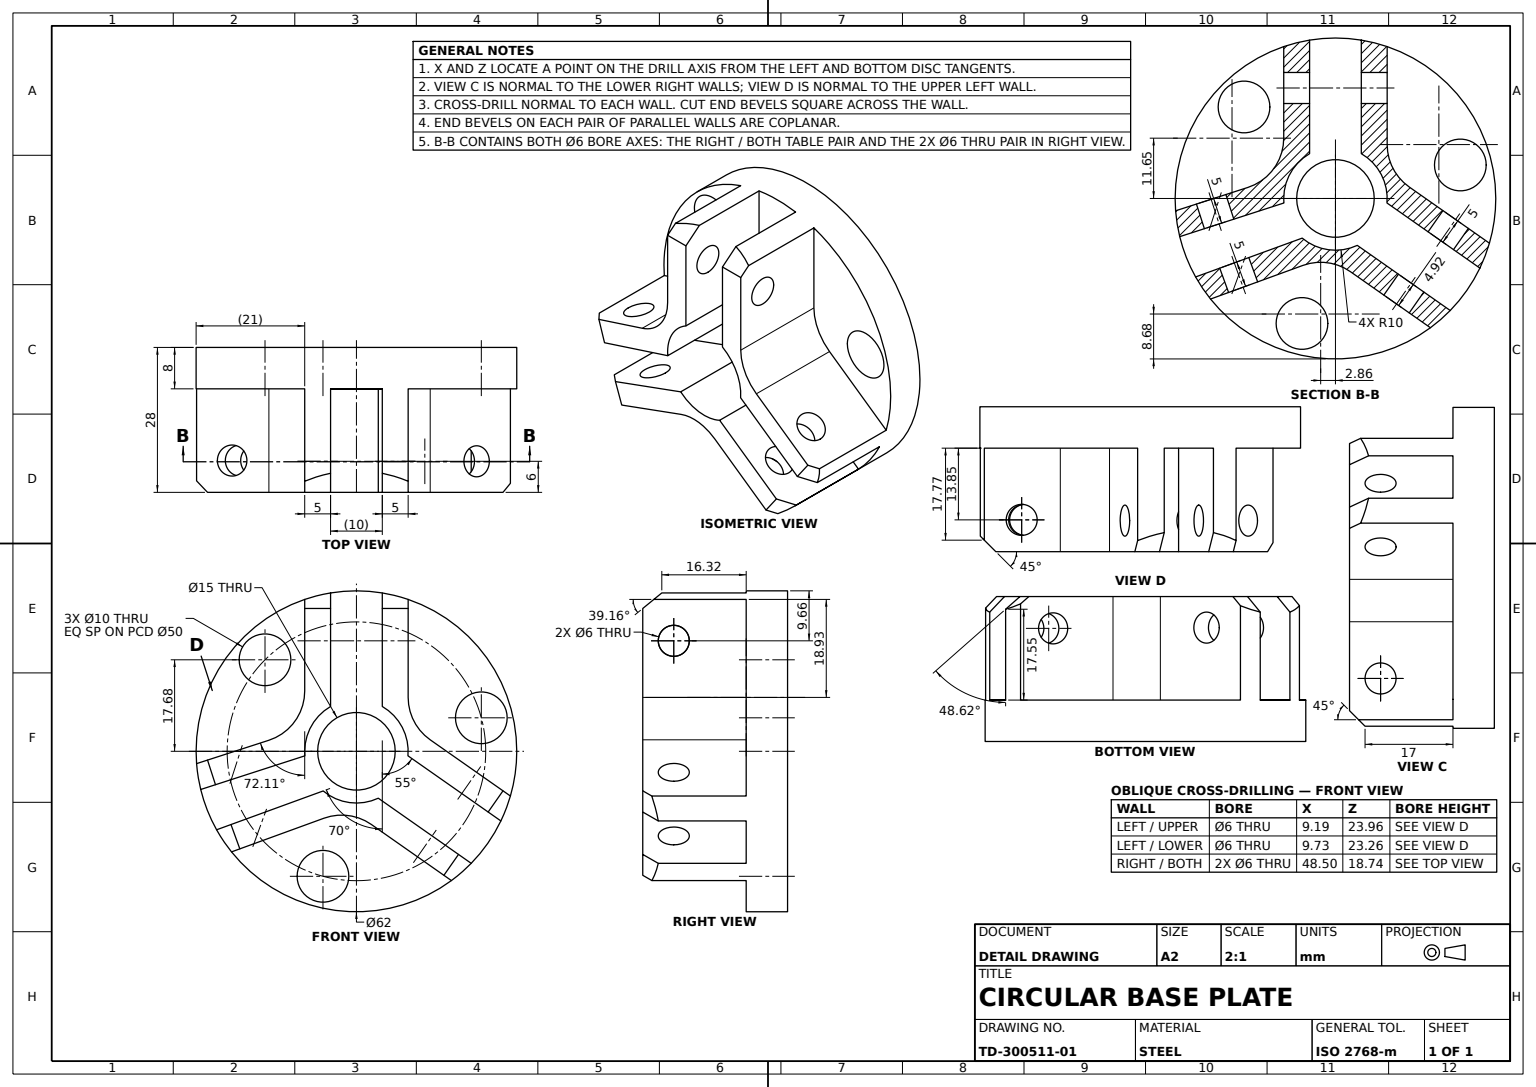
from build123d import *

# Parameters (mm, degrees)
BASE_DISC_SKETCH_R     = 31
BASE_DISC_62_DEPTH     = 8
SQUARE_CUT_SKETCH_R    = 5
SQUARE_CUT_10X10_DEPTH = 8
JAWS_DEPTH             = 20
JAW_NOTCH_1_DEPTH      = 10
JAW_NOTCH_2_DEPTH      = 10
JAW_NOTCH_3_DEPTH      = 10
JAW_NOTCH_4_DEPTH      = 10
JAW_NOTCH_5_DEPTH      = 10
JAW_NOTCH_6_DEPTH      = 10
JAW_HOLE_1_SKETCH_R    = 3
JAW_HOLE_1_6_DEPTH     = 10
JAW_HOLE_2_SKETCH_R    = 3
JAW_HOLE_2_6_DEPTH     = 10
JAW_HOLE_3_SKETCH_R    = 3
JAW_HOLE_3_6_DEPTH     = 10
JAW_START              = -10
JAW_HOLE_4_SKETCH_R    = 3
JAW_HOLE_4_6_DEPTH     = 10
JAW_HOLE_5_SKETCH_R    = 3
JAW_HOLE_5_6_DEPTH     = 10
JAW_HOLE_6_SKETCH_R    = 3
JAW_HOLE_6_6_DEPTH     = 10
HOLE_15_SKETCH_R       = 7.5
HOLE_15_DEPTH          = 10


with BuildPart() as part:
    # Base Disc Sketch → Base Disc Ø62 (new body)
    with BuildSketch(Plane.XY):
        Circle(BASE_DISC_SKETCH_R)
    extrude(amount=BASE_DISC_62_DEPTH)

    # Square Cut Sketch → Square Cut 10x10 (cut)
    with BuildSketch(Plane.XY.offset(8)):
        with Locations((-17.67766953, 17.67766953)):
            Circle(SQUARE_CUT_SKETCH_R)
        with Locations((24.148145657, 6.470476128)):
            Circle(SQUARE_CUT_SKETCH_R)
        with Locations((-6.470476128, -24.148145657)):
            Circle(SQUARE_CUT_SKETCH_R)
    extrude(amount=-SQUARE_CUT_10X10_DEPTH, mode=Mode.SUBTRACT)

    # Jaws Sketch → Jaws (add)
    with BuildSketch(Plane.XY.offset(8)):
        with BuildLine():
            Line((-30.109514993, -7.376795165), (-9.961946981, -0.871557427))
            ThreePointArc((-9.961946981, -0.871557427), (-9.990482216, 0.436193874), (-9.84807753, 1.736481777))
            ThreePointArc((-9.84807753, 1.736481777), (-8.191520443, 5.735764364), (-5, 8.660254038))
            Line((-5, 8.660254038), (-5, 10))
            Line((-5, 10), (-5, 30.594117082))
            ThreePointArc((-5, 30.594117082), (-7.526051267, 30.072554802), (-10, 29.342801502))
            Line((-10, 29.342801502), (-10, 11.649864154))
            ThreePointArc((-10, 11.649864154), (-11.915260032, 5.764545161), (-16.927395931, 2.133609416))
            Line((-16.927395931, 2.133609416), (-30.908458268, -2.38058973))
            ThreePointArc((-30.908458268, -2.38058973), (-30.611089207, -4.895019672), (-30.109514993, -7.376795165))
        make_face()
        with BuildLine():
            ThreePointArc((4.226182617, -9.06307787), (-1.305261922, -9.914448614), (-6.427876097, -7.660444431))
            Line((-6.427876097, -7.660444431), (-7.686825491, -8.118664537))
            Line((-7.686825491, -8.118664537), (-27.038965344, -15.162267413))
            ThreePointArc((-27.038965344, -15.162267413), (-25.684896703, -17.357594343), (-24.153012612, -19.432755383))
            Line((-24.153012612, -19.432755383), (-6.276119738, -12.926098496))
            ThreePointArc((-6.276119738, -12.926098496), (-1.550656383, -12.40857609), (2.879846058, -14.131504261))
            Line((2.879846058, -14.131504261), (18.365137045, -24.974421741))
            ThreePointArc((18.365137045, -24.974421741), (20.347505117, -23.387582934), (22.193351369, -21.64382487))
            Line((22.193351369, -21.64382487), (5.323638261, -9.831524585))
            Line((5.323638261, -9.831524585), (4.226182617, -9.06307787))
        make_face()
        with BuildLine():
            ThreePointArc((10, 29.342801502), (7.526051267, 30.072554802), (5, 30.594117082))
            Line((5, 30.594117082), (5, 10))
            Line((5, 10), (5, 8.660254038))
            ThreePointArc((5, 8.660254038), (8.870108332, 4.617486132), (9.961946981, -0.871557427))
            Line((9.961946981, -0.871557427), (11.059402625, -1.640004142))
            Line((11.059402625, -1.640004142), (27.929115732, -13.452304428))
            ThreePointArc((27.929115732, -13.452304428), (28.950760409, -11.083928535), (29.771980199, -8.638819075))
            Line((29.771980199, -8.638819075), (14.264235636, 2.219820568))
            ThreePointArc((14.264235636, 2.219820568), (11.129891668, 5.793854879), (10, 10.411341011))
            Line((10, 10.411341011), (10, 29.342801502))
        make_face()
    extrude(amount=JAWS_DEPTH)

    # Jaw Notch 1 Sketch → Jaw Notch 1 (cut)
    with BuildSketch(Plane.ZY.offset(-5)):
        Polygon((28, 30.594117082), (28, 27.594117082), (24.316442961, 30.594117082), align=None)
    extrude(amount=-JAW_NOTCH_1_DEPTH, mode=Mode.SUBTRACT)

    # Jaw Notch 2 Sketch → Jaw Notch 2 (cut)
    with BuildSketch(Plane(origin=(-5, 0, 0), x_dir=(0, 0, -1), z_dir=(1, 0, 0))):
        Polygon((-28, 30.594117082), (-24.316442961, 30.594117082), (-28, 27.594117082), align=None)
    extrude(amount=-JAW_NOTCH_2_DEPTH, mode=Mode.SUBTRACT)

    # Jaw Notch 3 Sketch → Jaw Notch 3 (cut)
    with BuildSketch(Plane(origin=(2.867882182, 4.095760221, 0), x_dir=(0.8191520442889944, -0.5735764363510426, 0), z_dir=(-0.5735764363510426, -0.8191520442889944, 0))):
        Polygon((30.594117082, 28), (30.594117082, 25), (27.594117082, 28), align=None)
    extrude(amount=-JAW_NOTCH_3_DEPTH, mode=Mode.SUBTRACT)

    # Jaw Notch 4 Sketch → Jaw Notch 4 (cut)
    with BuildSketch(Plane(origin=(-2.867882182, -4.095760221, 0), x_dir=(0.8191520442889944, -0.5735764363510426, 0), z_dir=(0.5735764363510426, 0.8191520442889944, 0))):
        Polygon((27.594117082, -28), (30.594117082, -28), (30.594117082, -25), align=None)
    extrude(amount=-JAW_NOTCH_4_DEPTH, mode=Mode.SUBTRACT)

    # Jaw Notch 5 Sketch → Jaw Notch 5 (cut)
    with BuildSketch(Plane(origin=(-0.685656401, 2.123567121, 0), x_dir=(0.9516254737982698, 0.3072604068509618, 0), z_dir=(0.3072604068509618, -0.9516254737982698, 0))):
        Polygon((-30.919578554, 28), (-27.919578554, 28), (-30.919578554, 25), align=None)
    extrude(amount=-JAW_NOTCH_5_DEPTH, mode=Mode.SUBTRACT)

    # Jaw Notch 6 Sketch → Jaw Notch 6 (cut)
    with BuildSketch(Plane(origin=(1.710100717, -4.698463104, 0), x_dir=(0.9396926207859072, 0.34202014332567215, 0), z_dir=(-0.3420201433256721, 0.9396926207859071, 0))):
        Polygon((-27.635003822, -28), (-30.594117082, -25.550278158), (-30.594117082, -28), align=None)
    extrude(amount=-JAW_NOTCH_6_DEPTH, mode=Mode.SUBTRACT)

    # Jaw Hole 1 Sketch → Jaw Hole 1 Ø6 (cut)
    with BuildSketch(Plane(origin=(-0.685656401, 2.123567121, 0), x_dir=(0.9516254737982698, 0.3072604068509618, 0), z_dir=(0.3072604068509618, -0.9516254737982698, 0))):
        with Locations((-22.919578554, 21.853934113)):
            Circle(JAW_HOLE_1_SKETCH_R)
    extrude(amount=-JAW_HOLE_1_6_DEPTH, mode=Mode.SUBTRACT)

    # Jaw Hole 2 Sketch → Jaw Hole 2 Ø6 (cut)
    with BuildSketch(Plane(origin=(1.710100717, -4.698463104, 0), x_dir=(0.9396926207859072, 0.34202014332567215, 0), z_dir=(-0.3420201433256721, 0.9396926207859071, 0))):
        with Locations(Location((-22.638380403, -21.853934113, 0), (0, 0, 180))):
            Circle(JAW_HOLE_2_SKETCH_R)
    extrude(amount=-JAW_HOLE_2_6_DEPTH, mode=Mode.SUBTRACT)

    # Jaw Hole 3 Sketch → Jaw Hole 3 Ø6 (cut)
    with BuildSketch(Plane.ZY.offset(-5)):
        with Locations((22, 21.342801502)):
            Circle(JAW_HOLE_3_SKETCH_R)
    extrude(amount=-JAW_HOLE_3_6_DEPTH, mode=Mode.SUBTRACT)

    # Jaw Hole 4 Sketch → Jaw Hole 4 Ø6 (cut)
    with BuildSketch(Plane(origin=(-5, 0, 0), x_dir=(0, 0, -1), z_dir=(1, 0, 0)).offset(JAW_START)):
        with Locations(Location((-22, 21.342801502, 0), (0, 0, 180))):
            Circle(JAW_HOLE_4_SKETCH_R)
    extrude(amount=JAW_HOLE_4_6_DEPTH, mode=Mode.SUBTRACT)

    # Jaw Hole 5 Sketch → Jaw Hole 5 Ø6 (cut)
    with BuildSketch(Plane(origin=(2.867882182, 4.095760221, 0), x_dir=(0.8191520442889944, -0.5735764363510426, 0), z_dir=(-0.5735764363510426, -0.8191520442889944, 0))):
        with Locations((21.368579376, 22)):
            Circle(JAW_HOLE_5_SKETCH_R)
    extrude(amount=-JAW_HOLE_5_6_DEPTH, mode=Mode.SUBTRACT)

    # Jaw Hole 6 Sketch → Jaw Hole 6 Ø6 (cut)
    with BuildSketch(Plane(origin=(-2.867882182, -4.095760221, 0), x_dir=(0.8191520442889944, -0.5735764363510426, 0), z_dir=(0.5735764363510426, 0.8191520442889944, 0)).offset(JAW_START)):
        with Locations((21.368579376, -22)):
            Circle(JAW_HOLE_6_SKETCH_R)
    extrude(amount=JAW_HOLE_6_6_DEPTH, mode=Mode.SUBTRACT)

    # Hole Ø15 Sketch → Hole Ø15 (cut)
    with BuildSketch(Plane.XY.offset(8)):
        Circle(HOLE_15_SKETCH_R)
    extrude(amount=-HOLE_15_DEPTH, mode=Mode.SUBTRACT)


solid = part.part
